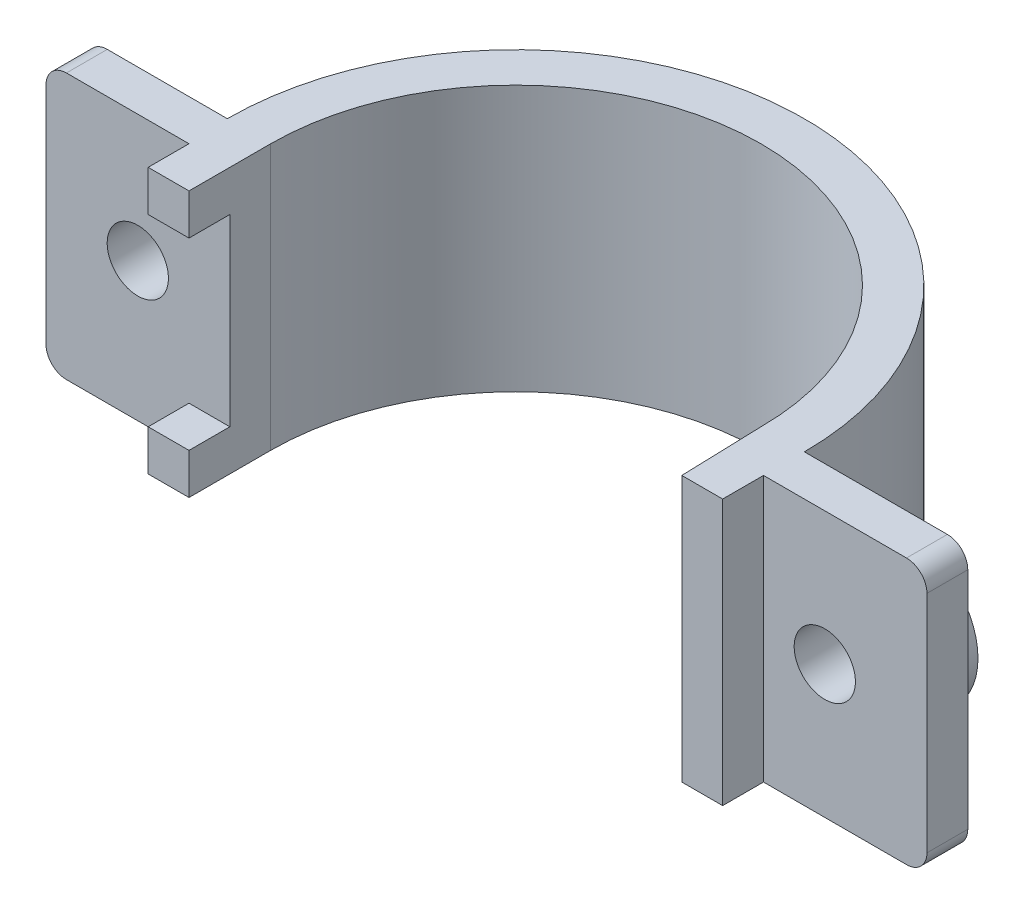
ISO-10303-21;
HEADER;
FILE_DESCRIPTION(('STEP AP214'),'2;1');
FILE_NAME('part.step','',(''),(''),'','','');
FILE_SCHEMA(('AUTOMOTIVE_DESIGN { 1 0 10303 214 1 1 1 1 }'));
ENDSEC;
DATA;
#1=APPLICATION_CONTEXT('core data for automotive mechanical design processes');
#2=APPLICATION_PROTOCOL_DEFINITION('international standard','automotive_design',2000,#1);
#3=PRODUCT_CONTEXT('',#1,'mechanical');
#4=PRODUCT('Part','Part','',(#3));
#5=PRODUCT_RELATED_PRODUCT_CATEGORY('part','',(#4));
#6=PRODUCT_DEFINITION_FORMATION('','',#4);
#7=PRODUCT_DEFINITION_CONTEXT('part definition',#1,'design');
#8=PRODUCT_DEFINITION('design','',#6,#7);
#9=PRODUCT_DEFINITION_SHAPE('','',#8);
#10=(LENGTH_UNIT() NAMED_UNIT(*) SI_UNIT(.MILLI.,.METRE.));
#11=(NAMED_UNIT(*) PLANE_ANGLE_UNIT() SI_UNIT($,.RADIAN.));
#12=(NAMED_UNIT(*) SI_UNIT($,.STERADIAN.) SOLID_ANGLE_UNIT());
#13=UNCERTAINTY_MEASURE_WITH_UNIT(LENGTH_MEASURE(1.E-05),#10,'distance_accuracy_value','');
#14=(GEOMETRIC_REPRESENTATION_CONTEXT(3) GLOBAL_UNCERTAINTY_ASSIGNED_CONTEXT((#13)) GLOBAL_UNIT_ASSIGNED_CONTEXT((#10,
#11,#12)) REPRESENTATION_CONTEXT('',''));
#15=CARTESIAN_POINT('',(0.,0.,0.));
#16=DIRECTION('',(0.,0.,1.));
#17=DIRECTION('',(1.,0.,0.));
#18=AXIS2_PLACEMENT_3D('',#15,#16,#17);
#19=CARTESIAN_POINT('',(165.624085247545,15.,0.));
#20=DIRECTION('',(0.,0.,1.));
#21=DIRECTION('',(1.,0.,0.));
#22=AXIS2_PLACEMENT_3D('',#19,#20,#21);
#23=PLANE('',#22);
#24=DIRECTION('',(1.,0.,0.));
#25=VECTOR('',#24,1.);
#26=CARTESIAN_POINT('',(130.624085247545,60.,0.));
#27=LINE('',#26,#25);
#28=CARTESIAN_POINT('',(130.624085247545,60.,0.));
#29=VERTEX_POINT('',#28);
#30=CARTESIAN_POINT('',(145.624085247545,60.,0.));
#31=VERTEX_POINT('',#30);
#32=EDGE_CURVE('E270',#29,#31,#27,.T.);
#33=ORIENTED_EDGE('',*,*,#32,.F.);
#34=DIRECTION('',(0.,1.,0.));
#35=VECTOR('',#34,1.);
#36=CARTESIAN_POINT('',(130.624085247545,9.99999999999999,0.));
#37=LINE('',#36,#35);
#38=CARTESIAN_POINT('',(130.624085247545,75.,0.));
#39=VERTEX_POINT('',#38);
#40=EDGE_CURVE('E364',#29,#39,#37,.T.);
#41=ORIENTED_EDGE('',*,*,#40,.T.);
#42=DIRECTION('',(-1.,0.,0.));
#43=VECTOR('',#42,1.);
#44=CARTESIAN_POINT('',(130.624085247545,75.,0.));
#45=LINE('',#44,#43);
#46=CARTESIAN_POINT('',(165.624085247545,75.,0.));
#47=VERTEX_POINT('',#46);
#48=EDGE_CURVE('E304',#47,#39,#45,.T.);
#49=ORIENTED_EDGE('',*,*,#48,.F.);
#50=CARTESIAN_POINT('',(165.624085247545,70.,0.));
#51=DIRECTION('',(0.,0.,1.));
#52=DIRECTION('',(1.,0.,0.));
#53=AXIS2_PLACEMENT_3D('',#50,#51,#52);
#54=CIRCLE('',#53,5.00000000000002);
#55=CARTESIAN_POINT('',(170.624085247545,70.,0.));
#56=VERTEX_POINT('',#55);
#57=EDGE_CURVE('E321',#56,#47,#54,.T.);
#58=ORIENTED_EDGE('',*,*,#57,.F.);
#59=DIRECTION('',(0.,1.,0.));
#60=VECTOR('',#59,1.);
#61=CARTESIAN_POINT('',(170.624085247545,70.,0.));
#62=LINE('',#61,#60);
#63=CARTESIAN_POINT('',(170.624085247545,15.,0.));
#64=VERTEX_POINT('',#63);
#65=EDGE_CURVE('E318',#64,#56,#62,.T.);
#66=ORIENTED_EDGE('',*,*,#65,.F.);
#67=CARTESIAN_POINT('',(165.624085247545,15.,0.));
#68=DIRECTION('',(0.,0.,1.));
#69=DIRECTION('',(1.,0.,0.));
#70=AXIS2_PLACEMENT_3D('',#67,#68,#69);
#71=CIRCLE('',#70,5.);
#72=CARTESIAN_POINT('',(165.624085247545,9.99999999999999,0.));
#73=VERTEX_POINT('',#72);
#74=EDGE_CURVE('E319',#73,#64,#71,.T.);
#75=ORIENTED_EDGE('',*,*,#74,.F.);
#76=DIRECTION('',(1.,0.,0.));
#77=VECTOR('',#76,1.);
#78=CARTESIAN_POINT('',(130.624085247545,9.99999999999999,0.));
#79=LINE('',#78,#77);
#80=CARTESIAN_POINT('',(130.624085247545,9.99999999999999,0.));
#81=VERTEX_POINT('',#80);
#82=EDGE_CURVE('E297',#81,#73,#79,.T.);
#83=ORIENTED_EDGE('',*,*,#82,.F.);
#84=CARTESIAN_POINT('',(130.624085247545,25.,0.));
#85=VERTEX_POINT('',#84);
#86=EDGE_CURVE('E374',#81,#85,#37,.T.);
#87=ORIENTED_EDGE('',*,*,#86,.T.);
#88=DIRECTION('',(-1.,0.,0.));
#89=VECTOR('',#88,1.);
#90=CARTESIAN_POINT('',(130.624085247545,25.,0.));
#91=LINE('',#90,#89);
#92=CARTESIAN_POINT('',(145.624085247545,25.,0.));
#93=VERTEX_POINT('',#92);
#94=EDGE_CURVE('E280',#93,#85,#91,.T.);
#95=ORIENTED_EDGE('',*,*,#94,.F.);
#96=CARTESIAN_POINT('',(145.624085247545,42.5,0.));
#97=DIRECTION('',(0.,0.,-1.));
#98=DIRECTION('',(-1.,0.,0.));
#99=AXIS2_PLACEMENT_3D('',#96,#97,#98);
#100=CIRCLE('',#99,17.5);
#101=EDGE_CURVE('E67',#31,#93,#100,.T.);
#102=ORIENTED_EDGE('',*,*,#101,.F.);
#103=EDGE_LOOP('',(#33,#41,#49,#58,#66,#75,#83,#87,#95,#102));
#104=FACE_BOUND('',#103,.T.);
#105=ADVANCED_FACE('F50',(#104),#23,.F.);
#106=CARTESIAN_POINT('',(-40.,15.,10.));
#107=DIRECTION('',(0.,0.,1.));
#108=DIRECTION('',(1.,0.,0.));
#109=AXIS2_PLACEMENT_3D('',#106,#107,#108);
#110=PLANE('',#109);
#111=CARTESIAN_POINT('',(-22.530823522442,43.9464892567154,10.));
#112=DIRECTION('',(0.,0.,-1.));
#113=DIRECTION('',(-1.,0.,0.));
#114=AXIS2_PLACEMENT_3D('',#111,#112,#113);
#115=CIRCLE('',#114,7.5);
#116=CARTESIAN_POINT('',(-30.030823522442,43.9464892567154,10.));
#117=VERTEX_POINT('',#116);
#118=EDGE_CURVE('E631',#117,#117,#115,.T.);
#119=ORIENTED_EDGE('',*,*,#118,.T.);
#120=EDGE_LOOP('',(#119));
#121=FACE_BOUND('',#120,.T.);
#122=DIRECTION('',(0.,-1.,0.));
#123=VECTOR('',#122,1.);
#124=CARTESIAN_POINT('',(-10.,20.,10.));
#125=LINE('',#124,#123);
#126=CARTESIAN_POINT('',(-10.,20.,10.));
#127=VERTEX_POINT('',#126);
#128=CARTESIAN_POINT('',(-10.,10.,10.));
#129=VERTEX_POINT('',#128);
#130=EDGE_CURVE('E382',#127,#129,#125,.T.);
#131=ORIENTED_EDGE('',*,*,#130,.F.);
#132=DIRECTION('',(-1.,0.,0.));
#133=VECTOR('',#132,1.);
#134=CARTESIAN_POINT('',(0.,20.,10.));
#135=LINE('',#134,#133);
#136=CARTESIAN_POINT('',(0.,20.,10.));
#137=VERTEX_POINT('',#136);
#138=EDGE_CURVE('E369',#137,#127,#135,.T.);
#139=ORIENTED_EDGE('',*,*,#138,.F.);
#140=DIRECTION('',(0.,1.,0.));
#141=VECTOR('',#140,1.);
#142=CARTESIAN_POINT('',(0.,75.,10.));
#143=LINE('',#142,#141);
#144=CARTESIAN_POINT('',(0.,65.,10.));
#145=VERTEX_POINT('',#144);
#146=EDGE_CURVE('E422',#137,#145,#143,.T.);
#147=ORIENTED_EDGE('',*,*,#146,.T.);
#148=DIRECTION('',(1.,0.,0.));
#149=VECTOR('',#148,1.);
#150=CARTESIAN_POINT('',(-10.,65.,10.));
#151=LINE('',#150,#149);
#152=CARTESIAN_POINT('',(-10.,65.,10.));
#153=VERTEX_POINT('',#152);
#154=EDGE_CURVE('E405',#153,#145,#151,.T.);
#155=ORIENTED_EDGE('',*,*,#154,.F.);
#156=DIRECTION('',(0.,-1.,0.));
#157=VECTOR('',#156,1.);
#158=CARTESIAN_POINT('',(-10.,75.,10.));
#159=LINE('',#158,#157);
#160=CARTESIAN_POINT('',(-10.,75.,10.));
#161=VERTEX_POINT('',#160);
#162=EDGE_CURVE('E396',#161,#153,#159,.T.);
#163=ORIENTED_EDGE('',*,*,#162,.F.);
#164=DIRECTION('',(-1.,0.,0.));
#165=VECTOR('',#164,1.);
#166=CARTESIAN_POINT('',(0.,75.,10.));
#167=LINE('',#166,#165);
#168=CARTESIAN_POINT('',(-40.,75.,10.));
#169=VERTEX_POINT('',#168);
#170=EDGE_CURVE('E425',#161,#169,#167,.T.);
#171=ORIENTED_EDGE('',*,*,#170,.T.);
#172=CARTESIAN_POINT('',(-40.,70.,10.));
#173=DIRECTION('',(0.,0.,1.));
#174=DIRECTION('',(1.,0.,0.));
#175=AXIS2_PLACEMENT_3D('',#172,#173,#174);
#176=CIRCLE('',#175,5.);
#177=CARTESIAN_POINT('',(-45.,70.,10.));
#178=VERTEX_POINT('',#177);
#179=EDGE_CURVE('E430',#169,#178,#176,.T.);
#180=ORIENTED_EDGE('',*,*,#179,.T.);
#181=DIRECTION('',(0.,-1.,0.));
#182=VECTOR('',#181,1.);
#183=CARTESIAN_POINT('',(-45.,70.,10.));
#184=LINE('',#183,#182);
#185=CARTESIAN_POINT('',(-45.,15.,10.));
#186=VERTEX_POINT('',#185);
#187=EDGE_CURVE('E429',#178,#186,#184,.T.);
#188=ORIENTED_EDGE('',*,*,#187,.T.);
#189=CARTESIAN_POINT('',(-40.,15.,10.));
#190=DIRECTION('',(0.,0.,1.));
#191=DIRECTION('',(1.,0.,0.));
#192=AXIS2_PLACEMENT_3D('',#189,#190,#191);
#193=CIRCLE('',#192,5.);
#194=CARTESIAN_POINT('',(-40.,10.,10.));
#195=VERTEX_POINT('',#194);
#196=EDGE_CURVE('E431',#186,#195,#193,.T.);
#197=ORIENTED_EDGE('',*,*,#196,.T.);
#198=DIRECTION('',(1.,0.,0.));
#199=VECTOR('',#198,1.);
#200=CARTESIAN_POINT('',(0.,10.,10.));
#201=LINE('',#200,#199);
#202=EDGE_CURVE('E433',#195,#129,#201,.T.);
#203=ORIENTED_EDGE('',*,*,#202,.T.);
#204=EDGE_LOOP('',(#131,#139,#147,#155,#163,#171,#180,#188,#197,#203));
#205=FACE_BOUND('',#204,.T.);
#206=ADVANCED_FACE('F482',(#121,#205),#110,.T.);
#207=CARTESIAN_POINT('',(0.,75.,10.));
#208=DIRECTION('',(-1.,0.,0.));
#209=DIRECTION('',(0.,0.,1.));
#210=AXIS2_PLACEMENT_3D('',#207,#208,#209);
#211=PLANE('',#210);
#212=DIRECTION('',(0.,1.,0.));
#213=VECTOR('',#212,1.);
#214=CARTESIAN_POINT('',(0.,75.,0.));
#215=LINE('',#214,#213);
#216=CARTESIAN_POINT('',(0.,9.99999999999999,0.));
#217=VERTEX_POINT('',#216);
#218=CARTESIAN_POINT('',(0.,75.,0.));
#219=VERTEX_POINT('',#218);
#220=EDGE_CURVE('E423',#217,#219,#215,.T.);
#221=ORIENTED_EDGE('',*,*,#220,.T.);
#222=DIRECTION('',(0.,0.,-1.));
#223=VECTOR('',#222,1.);
#224=CARTESIAN_POINT('',(0.,75.,10.));
#225=LINE('',#224,#223);
#226=CARTESIAN_POINT('',(0.,75.,20.));
#227=VERTEX_POINT('',#226);
#228=EDGE_CURVE('E11',#227,#219,#225,.T.);
#229=ORIENTED_EDGE('',*,*,#228,.F.);
#230=DIRECTION('',(0.,1.,0.));
#231=VECTOR('',#230,1.);
#232=CARTESIAN_POINT('',(0.,65.,20.));
#233=LINE('',#232,#231);
#234=CARTESIAN_POINT('',(0.,65.,20.));
#235=VERTEX_POINT('',#234);
#236=EDGE_CURVE('E400',#235,#227,#233,.T.);
#237=ORIENTED_EDGE('',*,*,#236,.F.);
#238=DIRECTION('',(0.,0.,-1.));
#239=VECTOR('',#238,1.);
#240=CARTESIAN_POINT('',(0.,65.,20.));
#241=LINE('',#240,#239);
#242=EDGE_CURVE('E410',#235,#145,#241,.T.);
#243=ORIENTED_EDGE('',*,*,#242,.T.);
#244=ORIENTED_EDGE('',*,*,#146,.F.);
#245=DIRECTION('',(0.,0.,-1.));
#246=VECTOR('',#245,1.);
#247=CARTESIAN_POINT('',(0.,20.,20.));
#248=LINE('',#247,#246);
#249=CARTESIAN_POINT('',(0.,20.,20.));
#250=VERTEX_POINT('',#249);
#251=EDGE_CURVE('E392',#250,#137,#248,.T.);
#252=ORIENTED_EDGE('',*,*,#251,.F.);
#253=DIRECTION('',(0.,1.,0.));
#254=VECTOR('',#253,1.);
#255=CARTESIAN_POINT('',(0.,10.,20.));
#256=LINE('',#255,#254);
#257=CARTESIAN_POINT('',(0.,10.,20.));
#258=VERTEX_POINT('',#257);
#259=EDGE_CURVE('E379',#258,#250,#256,.T.);
#260=ORIENTED_EDGE('',*,*,#259,.F.);
#261=DIRECTION('',(0.,0.,-1.));
#262=VECTOR('',#261,1.);
#263=CARTESIAN_POINT('',(0.,10.,10.));
#264=LINE('',#263,#262);
#265=EDGE_CURVE('E436',#258,#217,#264,.T.);
#266=ORIENTED_EDGE('',*,*,#265,.T.);
#267=EDGE_LOOP('',(#221,#229,#237,#243,#244,#252,#260,#266));
#268=FACE_BOUND('',#267,.T.);
#269=ADVANCED_FACE('F47',(#268),#211,.F.);
#270=CARTESIAN_POINT('',(0.,75.,10.));
#271=DIRECTION('',(0.,-1.,0.));
#272=DIRECTION('',(0.,0.,-1.));
#273=AXIS2_PLACEMENT_3D('',#270,#271,#272);
#274=PLANE('',#273);
#275=ORIENTED_EDGE('',*,*,#228,.T.);
#276=CARTESIAN_POINT('',(60.,75.,0.));
#277=DIRECTION('',(0.,1.,0.));
#278=DIRECTION('',(0.,0.,1.));
#279=AXIS2_PLACEMENT_3D('',#276,#277,#278);
#280=CIRCLE('',#279,60.);
#281=CARTESIAN_POINT('',(120.,75.,0.));
#282=VERTEX_POINT('',#281);
#283=EDGE_CURVE('E365',#282,#219,#280,.T.);
#284=ORIENTED_EDGE('',*,*,#283,.F.);
#285=DIRECTION('',(0.0311890815739658,0.,0.999513502255259));
#286=VECTOR('',#285,1.);
#287=CARTESIAN_POINT('',(120.624085247545,75.,20.));
#288=LINE('',#287,#286);
#289=CARTESIAN_POINT('',(120.624085247545,75.,20.));
#290=VERTEX_POINT('',#289);
#291=EDGE_CURVE('E340',#282,#290,#288,.T.);
#292=ORIENTED_EDGE('',*,*,#291,.T.);
#293=DIRECTION('',(1.,0.,0.));
#294=VECTOR('',#293,1.);
#295=CARTESIAN_POINT('',(130.624085247545,75.,20.));
#296=LINE('',#295,#294);
#297=CARTESIAN_POINT('',(130.624085247545,75.,20.));
#298=VERTEX_POINT('',#297);
#299=EDGE_CURVE('E347',#290,#298,#296,.T.);
#300=ORIENTED_EDGE('',*,*,#299,.T.);
#301=DIRECTION('',(0.,0.,-1.));
#302=VECTOR('',#301,1.);
#303=CARTESIAN_POINT('',(130.624085247545,75.,0.));
#304=LINE('',#303,#302);
#305=CARTESIAN_POINT('',(130.624085247545,75.,10.));
#306=VERTEX_POINT('',#305);
#307=EDGE_CURVE('E341',#298,#306,#304,.T.);
#308=ORIENTED_EDGE('',*,*,#307,.T.);
#309=DIRECTION('',(-1.,0.,0.));
#310=VECTOR('',#309,1.);
#311=CARTESIAN_POINT('',(130.624085247545,75.,10.));
#312=LINE('',#311,#310);
#313=CARTESIAN_POINT('',(165.624085247545,75.,10.));
#314=VERTEX_POINT('',#313);
#315=EDGE_CURVE('E312',#314,#306,#312,.T.);
#316=ORIENTED_EDGE('',*,*,#315,.F.);
#317=DIRECTION('',(0.,0.,-1.));
#318=VECTOR('',#317,1.);
#319=CARTESIAN_POINT('',(165.624085247545,75.,10.));
#320=LINE('',#319,#318);
#321=EDGE_CURVE('E317',#314,#47,#320,.T.);
#322=ORIENTED_EDGE('',*,*,#321,.T.);
#323=ORIENTED_EDGE('',*,*,#48,.T.);
#324=CARTESIAN_POINT('',(60.,75.,0.));
#325=DIRECTION('',(0.,1.,0.));
#326=DIRECTION('',(0.,0.,1.));
#327=AXIS2_PLACEMENT_3D('',#324,#325,#326);
#328=CIRCLE('',#327,70.6240852475448);
#329=CARTESIAN_POINT('',(-10.6240852475448,75.,0.));
#330=VERTEX_POINT('',#329);
#331=EDGE_CURVE('E357',#39,#330,#328,.T.);
#332=ORIENTED_EDGE('',*,*,#331,.T.);
#333=DIRECTION('',(-1.,0.,0.));
#334=VECTOR('',#333,1.);
#335=CARTESIAN_POINT('',(0.,75.,0.));
#336=LINE('',#335,#334);
#337=CARTESIAN_POINT('',(-40.,75.,0.));
#338=VERTEX_POINT('',#337);
#339=EDGE_CURVE('E437',#330,#338,#336,.T.);
#340=ORIENTED_EDGE('',*,*,#339,.T.);
#341=DIRECTION('',(0.,0.,-1.));
#342=VECTOR('',#341,1.);
#343=CARTESIAN_POINT('',(-40.,75.,10.));
#344=LINE('',#343,#342);
#345=EDGE_CURVE('E54',#169,#338,#344,.T.);
#346=ORIENTED_EDGE('',*,*,#345,.F.);
#347=ORIENTED_EDGE('',*,*,#170,.F.);
#348=DIRECTION('',(0.,0.,-1.));
#349=VECTOR('',#348,1.);
#350=CARTESIAN_POINT('',(-10.,75.,20.));
#351=LINE('',#350,#349);
#352=CARTESIAN_POINT('',(-10.,75.,20.));
#353=VERTEX_POINT('',#352);
#354=EDGE_CURVE('E420',#353,#161,#351,.T.);
#355=ORIENTED_EDGE('',*,*,#354,.F.);
#356=DIRECTION('',(-1.,0.,0.));
#357=VECTOR('',#356,1.);
#358=CARTESIAN_POINT('',(0.,75.,20.));
#359=LINE('',#358,#357);
#360=EDGE_CURVE('E402',#227,#353,#359,.T.);
#361=ORIENTED_EDGE('',*,*,#360,.F.);
#362=EDGE_LOOP('',(#275,#284,#292,#300,#308,#316,#322,#323,#332,#340,#346,#347,#355,#361));
#363=FACE_BOUND('',#362,.T.);
#364=ADVANCED_FACE('F487',(#363),#274,.F.);
#365=CARTESIAN_POINT('',(-40.,70.,10.));
#366=DIRECTION('',(0.,0.,-1.));
#367=DIRECTION('',(-1.,0.,0.));
#368=AXIS2_PLACEMENT_3D('',#365,#366,#367);
#369=CYLINDRICAL_SURFACE('',#368,5.);
#370=CARTESIAN_POINT('',(-40.,70.,0.));
#371=DIRECTION('',(0.,0.,1.));
#372=DIRECTION('',(1.,0.,0.));
#373=AXIS2_PLACEMENT_3D('',#370,#371,#372);
#374=CIRCLE('',#373,5.);
#375=CARTESIAN_POINT('',(-45.,70.,0.));
#376=VERTEX_POINT('',#375);
#377=EDGE_CURVE('E441',#338,#376,#374,.T.);
#378=ORIENTED_EDGE('',*,*,#377,.T.);
#379=DIRECTION('',(0.,0.,-1.));
#380=VECTOR('',#379,1.);
#381=CARTESIAN_POINT('',(-45.,70.,10.));
#382=LINE('',#381,#380);
#383=EDGE_CURVE('E460',#178,#376,#382,.T.);
#384=ORIENTED_EDGE('',*,*,#383,.F.);
#385=ORIENTED_EDGE('',*,*,#179,.F.);
#386=ORIENTED_EDGE('',*,*,#345,.T.);
#387=EDGE_LOOP('',(#378,#384,#385,#386));
#388=FACE_BOUND('',#387,.T.);
#389=ADVANCED_FACE('F463',(#388),#369,.T.);
#390=CARTESIAN_POINT('',(-45.,70.,10.));
#391=DIRECTION('',(1.,0.,0.));
#392=DIRECTION('',(0.,0.,-1.));
#393=AXIS2_PLACEMENT_3D('',#390,#391,#392);
#394=PLANE('',#393);
#395=DIRECTION('',(0.,-1.,0.));
#396=VECTOR('',#395,1.);
#397=CARTESIAN_POINT('',(-45.,70.,0.));
#398=LINE('',#397,#396);
#399=CARTESIAN_POINT('',(-45.,15.,0.));
#400=VERTEX_POINT('',#399);
#401=EDGE_CURVE('E442',#376,#400,#398,.T.);
#402=ORIENTED_EDGE('',*,*,#401,.T.);
#403=DIRECTION('',(0.,0.,-1.));
#404=VECTOR('',#403,1.);
#405=CARTESIAN_POINT('',(-45.,15.,10.));
#406=LINE('',#405,#404);
#407=EDGE_CURVE('E453',#186,#400,#406,.T.);
#408=ORIENTED_EDGE('',*,*,#407,.F.);
#409=ORIENTED_EDGE('',*,*,#187,.F.);
#410=ORIENTED_EDGE('',*,*,#383,.T.);
#411=EDGE_LOOP('',(#402,#408,#409,#410));
#412=FACE_BOUND('',#411,.T.);
#413=ADVANCED_FACE('F478',(#412),#394,.F.);
#414=CARTESIAN_POINT('',(-40.,15.,10.));
#415=DIRECTION('',(0.,0.,-1.));
#416=DIRECTION('',(-1.,0.,0.));
#417=AXIS2_PLACEMENT_3D('',#414,#415,#416);
#418=CYLINDRICAL_SURFACE('',#417,5.);
#419=CARTESIAN_POINT('',(-40.,15.,0.));
#420=DIRECTION('',(0.,0.,1.));
#421=DIRECTION('',(1.,0.,0.));
#422=AXIS2_PLACEMENT_3D('',#419,#420,#421);
#423=CIRCLE('',#422,5.);
#424=CARTESIAN_POINT('',(-40.,10.,0.));
#425=VERTEX_POINT('',#424);
#426=EDGE_CURVE('E444',#400,#425,#423,.T.);
#427=ORIENTED_EDGE('',*,*,#426,.T.);
#428=DIRECTION('',(0.,0.,-1.));
#429=VECTOR('',#428,1.);
#430=CARTESIAN_POINT('',(-40.,10.,10.));
#431=LINE('',#430,#429);
#432=EDGE_CURVE('E454',#195,#425,#431,.T.);
#433=ORIENTED_EDGE('',*,*,#432,.F.);
#434=ORIENTED_EDGE('',*,*,#196,.F.);
#435=ORIENTED_EDGE('',*,*,#407,.T.);
#436=EDGE_LOOP('',(#427,#433,#434,#435));
#437=FACE_BOUND('',#436,.T.);
#438=ADVANCED_FACE('F477',(#437),#418,.T.);
#439=CARTESIAN_POINT('',(0.,10.,10.));
#440=DIRECTION('',(0.,1.,0.));
#441=DIRECTION('',(0.,0.,1.));
#442=AXIS2_PLACEMENT_3D('',#439,#440,#441);
#443=PLANE('',#442);
#444=DIRECTION('',(1.,0.,0.));
#445=VECTOR('',#444,1.);
#446=CARTESIAN_POINT('',(0.,10.,0.));
#447=LINE('',#446,#445);
#448=CARTESIAN_POINT('',(-10.6240852475448,9.99999999999999,0.));
#449=VERTEX_POINT('',#448);
#450=EDGE_CURVE('E424',#425,#449,#447,.T.);
#451=ORIENTED_EDGE('',*,*,#450,.T.);
#452=CARTESIAN_POINT('',(60.,9.99999999999999,0.));
#453=DIRECTION('',(0.,1.,0.));
#454=DIRECTION('',(0.,0.,1.));
#455=AXIS2_PLACEMENT_3D('',#452,#453,#454);
#456=CIRCLE('',#455,70.6240852475448);
#457=EDGE_CURVE('E360',#81,#449,#456,.T.);
#458=ORIENTED_EDGE('',*,*,#457,.F.);
#459=ORIENTED_EDGE('',*,*,#82,.T.);
#460=DIRECTION('',(0.,0.,-1.));
#461=VECTOR('',#460,1.);
#462=CARTESIAN_POINT('',(165.624085247545,9.99999999999999,10.));
#463=LINE('',#462,#461);
#464=CARTESIAN_POINT('',(165.624085247545,9.99999999999999,10.));
#465=VERTEX_POINT('',#464);
#466=EDGE_CURVE('E333',#465,#73,#463,.T.);
#467=ORIENTED_EDGE('',*,*,#466,.F.);
#468=DIRECTION('',(1.,0.,0.));
#469=VECTOR('',#468,1.);
#470=CARTESIAN_POINT('',(130.624085247545,9.99999999999999,10.));
#471=LINE('',#470,#469);
#472=CARTESIAN_POINT('',(130.624085247545,9.99999999999999,10.));
#473=VERTEX_POINT('',#472);
#474=EDGE_CURVE('E302',#473,#465,#471,.T.);
#475=ORIENTED_EDGE('',*,*,#474,.F.);
#476=DIRECTION('',(0.,0.,-1.));
#477=VECTOR('',#476,1.);
#478=CARTESIAN_POINT('',(130.624085247545,9.99999999999999,0.));
#479=LINE('',#478,#477);
#480=CARTESIAN_POINT('',(130.624085247545,9.99999999999999,20.));
#481=VERTEX_POINT('',#480);
#482=EDGE_CURVE('E342',#481,#473,#479,.T.);
#483=ORIENTED_EDGE('',*,*,#482,.F.);
#484=DIRECTION('',(1.,0.,0.));
#485=VECTOR('',#484,1.);
#486=CARTESIAN_POINT('',(130.624085247545,9.99999999999999,20.));
#487=LINE('',#486,#485);
#488=CARTESIAN_POINT('',(120.624085247545,9.99999999999999,20.));
#489=VERTEX_POINT('',#488);
#490=EDGE_CURVE('E344',#489,#481,#487,.T.);
#491=ORIENTED_EDGE('',*,*,#490,.F.);
#492=DIRECTION('',(0.0311890815739658,0.,0.999513502255259));
#493=VECTOR('',#492,1.);
#494=CARTESIAN_POINT('',(120.624085247545,9.99999999999999,20.));
#495=LINE('',#494,#493);
#496=CARTESIAN_POINT('',(120.,9.99999999999999,0.));
#497=VERTEX_POINT('',#496);
#498=EDGE_CURVE('E336',#497,#489,#495,.T.);
#499=ORIENTED_EDGE('',*,*,#498,.F.);
#500=CARTESIAN_POINT('',(60.,9.99999999999999,0.));
#501=DIRECTION('',(0.,1.,0.));
#502=DIRECTION('',(0.,0.,1.));
#503=AXIS2_PLACEMENT_3D('',#500,#501,#502);
#504=CIRCLE('',#503,60.);
#505=EDGE_CURVE('E363',#497,#217,#504,.T.);
#506=ORIENTED_EDGE('',*,*,#505,.T.);
#507=ORIENTED_EDGE('',*,*,#265,.F.);
#508=DIRECTION('',(1.,0.,0.));
#509=VECTOR('',#508,1.);
#510=CARTESIAN_POINT('',(-10.,10.,20.));
#511=LINE('',#510,#509);
#512=CARTESIAN_POINT('',(-10.,10.,20.));
#513=VERTEX_POINT('',#512);
#514=EDGE_CURVE('E380',#513,#258,#511,.T.);
#515=ORIENTED_EDGE('',*,*,#514,.F.);
#516=DIRECTION('',(0.,0.,-1.));
#517=VECTOR('',#516,1.);
#518=CARTESIAN_POINT('',(-10.,10.,20.));
#519=LINE('',#518,#517);
#520=EDGE_CURVE('E386',#513,#129,#519,.T.);
#521=ORIENTED_EDGE('',*,*,#520,.T.);
#522=ORIENTED_EDGE('',*,*,#202,.F.);
#523=ORIENTED_EDGE('',*,*,#432,.T.);
#524=EDGE_LOOP('',(#451,#458,#459,#467,#475,#483,#491,#499,#506,#507,#515,#521,#522,#523));
#525=FACE_BOUND('',#524,.T.);
#526=ADVANCED_FACE('F512',(#525),#443,.F.);
#527=CARTESIAN_POINT('',(-40.,15.,0.));
#528=DIRECTION('',(0.,0.,1.));
#529=DIRECTION('',(1.,0.,0.));
#530=AXIS2_PLACEMENT_3D('',#527,#528,#529);
#531=PLANE('',#530);
#532=DIRECTION('',(1.,0.,0.));
#533=VECTOR('',#532,1.);
#534=CARTESIAN_POINT('',(-10.6240852475448,60.,0.));
#535=LINE('',#534,#533);
#536=CARTESIAN_POINT('',(-20.6240852475448,60.,0.));
#537=VERTEX_POINT('',#536);
#538=CARTESIAN_POINT('',(-10.6240852475448,60.,0.));
#539=VERTEX_POINT('',#538);
#540=EDGE_CURVE('E61',#537,#539,#535,.T.);
#541=ORIENTED_EDGE('',*,*,#540,.F.);
#542=CARTESIAN_POINT('',(-20.6240852475448,42.5,0.));
#543=DIRECTION('',(0.,0.,-1.));
#544=DIRECTION('',(-1.,0.,0.));
#545=AXIS2_PLACEMENT_3D('',#542,#543,#544);
#546=CIRCLE('',#545,17.5);
#547=CARTESIAN_POINT('',(-20.6240852475448,25.,0.));
#548=VERTEX_POINT('',#547);
#549=EDGE_CURVE('E265',#548,#537,#546,.T.);
#550=ORIENTED_EDGE('',*,*,#549,.F.);
#551=DIRECTION('',(-1.,0.,0.));
#552=VECTOR('',#551,1.);
#553=CARTESIAN_POINT('',(-20.6240852475448,25.,0.));
#554=LINE('',#553,#552);
#555=CARTESIAN_POINT('',(-10.6240852475448,25.,0.));
#556=VERTEX_POINT('',#555);
#557=EDGE_CURVE('E543',#556,#548,#554,.T.);
#558=ORIENTED_EDGE('',*,*,#557,.F.);
#559=DIRECTION('',(0.,1.,0.));
#560=VECTOR('',#559,1.);
#561=CARTESIAN_POINT('',(-10.6240852475448,9.99999999999999,0.));
#562=LINE('',#561,#560);
#563=EDGE_CURVE('E371',#449,#556,#562,.T.);
#564=ORIENTED_EDGE('',*,*,#563,.F.);
#565=ORIENTED_EDGE('',*,*,#450,.F.);
#566=ORIENTED_EDGE('',*,*,#426,.F.);
#567=ORIENTED_EDGE('',*,*,#401,.F.);
#568=ORIENTED_EDGE('',*,*,#377,.F.);
#569=ORIENTED_EDGE('',*,*,#339,.F.);
#570=EDGE_CURVE('E372',#539,#330,#562,.T.);
#571=ORIENTED_EDGE('',*,*,#570,.F.);
#572=EDGE_LOOP('',(#541,#550,#558,#564,#565,#566,#567,#568,#569,#571));
#573=FACE_BOUND('',#572,.T.);
#574=ADVANCED_FACE('F474',(#573),#531,.F.);
#575=CARTESIAN_POINT('',(-10.,75.,20.));
#576=DIRECTION('',(1.,0.,0.));
#577=DIRECTION('',(0.,0.,-1.));
#578=AXIS2_PLACEMENT_3D('',#575,#576,#577);
#579=PLANE('',#578);
#580=ORIENTED_EDGE('',*,*,#162,.T.);
#581=DIRECTION('',(0.,0.,-1.));
#582=VECTOR('',#581,1.);
#583=CARTESIAN_POINT('',(-10.,65.,20.));
#584=LINE('',#583,#582);
#585=CARTESIAN_POINT('',(-10.,65.,20.));
#586=VERTEX_POINT('',#585);
#587=EDGE_CURVE('E412',#586,#153,#584,.T.);
#588=ORIENTED_EDGE('',*,*,#587,.F.);
#589=DIRECTION('',(0.,-1.,0.));
#590=VECTOR('',#589,1.);
#591=CARTESIAN_POINT('',(-10.,75.,20.));
#592=LINE('',#591,#590);
#593=EDGE_CURVE('E404',#353,#586,#592,.T.);
#594=ORIENTED_EDGE('',*,*,#593,.F.);
#595=ORIENTED_EDGE('',*,*,#354,.T.);
#596=EDGE_LOOP('',(#580,#588,#594,#595));
#597=FACE_BOUND('',#596,.T.);
#598=ADVANCED_FACE('F493',(#597),#579,.F.);
#599=CARTESIAN_POINT('',(-10.,65.,20.));
#600=DIRECTION('',(0.,1.,0.));
#601=DIRECTION('',(0.,0.,1.));
#602=AXIS2_PLACEMENT_3D('',#599,#600,#601);
#603=PLANE('',#602);
#604=ORIENTED_EDGE('',*,*,#154,.T.);
#605=ORIENTED_EDGE('',*,*,#242,.F.);
#606=DIRECTION('',(1.,0.,0.));
#607=VECTOR('',#606,1.);
#608=CARTESIAN_POINT('',(-10.,65.,20.));
#609=LINE('',#608,#607);
#610=EDGE_CURVE('E409',#586,#235,#609,.T.);
#611=ORIENTED_EDGE('',*,*,#610,.F.);
#612=ORIENTED_EDGE('',*,*,#587,.T.);
#613=EDGE_LOOP('',(#604,#605,#611,#612));
#614=FACE_BOUND('',#613,.T.);
#615=ADVANCED_FACE('F822',(#614),#603,.F.);
#616=CARTESIAN_POINT('',(0.,0.,20.));
#617=DIRECTION('',(0.,0.,1.));
#618=DIRECTION('',(1.,0.,0.));
#619=AXIS2_PLACEMENT_3D('',#616,#617,#618);
#620=PLANE('',#619);
#621=ORIENTED_EDGE('',*,*,#236,.T.);
#622=ORIENTED_EDGE('',*,*,#360,.T.);
#623=ORIENTED_EDGE('',*,*,#593,.T.);
#624=ORIENTED_EDGE('',*,*,#610,.T.);
#625=EDGE_LOOP('',(#621,#622,#623,#624));
#626=FACE_BOUND('',#625,.T.);
#627=ADVANCED_FACE('F492',(#626),#620,.T.);
#628=CARTESIAN_POINT('',(0.,20.,20.));
#629=DIRECTION('',(0.,-1.,0.));
#630=DIRECTION('',(0.,0.,-1.));
#631=AXIS2_PLACEMENT_3D('',#628,#629,#630);
#632=PLANE('',#631);
#633=ORIENTED_EDGE('',*,*,#138,.T.);
#634=DIRECTION('',(0.,0.,-1.));
#635=VECTOR('',#634,1.);
#636=CARTESIAN_POINT('',(-10.,20.,20.));
#637=LINE('',#636,#635);
#638=CARTESIAN_POINT('',(-10.,20.,20.));
#639=VERTEX_POINT('',#638);
#640=EDGE_CURVE('E391',#639,#127,#637,.T.);
#641=ORIENTED_EDGE('',*,*,#640,.F.);
#642=DIRECTION('',(-1.,0.,0.));
#643=VECTOR('',#642,1.);
#644=CARTESIAN_POINT('',(0.,20.,20.));
#645=LINE('',#644,#643);
#646=EDGE_CURVE('E384',#250,#639,#645,.T.);
#647=ORIENTED_EDGE('',*,*,#646,.F.);
#648=ORIENTED_EDGE('',*,*,#251,.T.);
#649=EDGE_LOOP('',(#633,#641,#647,#648));
#650=FACE_BOUND('',#649,.T.);
#651=ADVANCED_FACE('F806',(#650),#632,.F.);
#652=CARTESIAN_POINT('',(-10.,20.,20.));
#653=DIRECTION('',(1.,0.,0.));
#654=DIRECTION('',(0.,0.,-1.));
#655=AXIS2_PLACEMENT_3D('',#652,#653,#654);
#656=PLANE('',#655);
#657=ORIENTED_EDGE('',*,*,#130,.T.);
#658=ORIENTED_EDGE('',*,*,#520,.F.);
#659=DIRECTION('',(0.,-1.,0.));
#660=VECTOR('',#659,1.);
#661=CARTESIAN_POINT('',(-10.,20.,20.));
#662=LINE('',#661,#660);
#663=EDGE_CURVE('E383',#639,#513,#662,.T.);
#664=ORIENTED_EDGE('',*,*,#663,.F.);
#665=ORIENTED_EDGE('',*,*,#640,.T.);
#666=EDGE_LOOP('',(#657,#658,#664,#665));
#667=FACE_BOUND('',#666,.T.);
#668=ADVANCED_FACE('F796',(#667),#656,.F.);
#669=CARTESIAN_POINT('',(0.,0.,20.));
#670=DIRECTION('',(0.,0.,1.));
#671=DIRECTION('',(1.,0.,0.));
#672=AXIS2_PLACEMENT_3D('',#669,#670,#671);
#673=PLANE('',#672);
#674=ORIENTED_EDGE('',*,*,#514,.T.);
#675=ORIENTED_EDGE('',*,*,#259,.T.);
#676=ORIENTED_EDGE('',*,*,#646,.T.);
#677=ORIENTED_EDGE('',*,*,#663,.T.);
#678=EDGE_LOOP('',(#674,#675,#676,#677));
#679=FACE_BOUND('',#678,.T.);
#680=ADVANCED_FACE('F790',(#679),#673,.T.);
#681=CARTESIAN_POINT('',(60.,9.99999999999999,0.));
#682=DIRECTION('',(0.,1.,0.));
#683=DIRECTION('',(0.,0.,1.));
#684=AXIS2_PLACEMENT_3D('',#681,#682,#683);
#685=CYLINDRICAL_SURFACE('',#684,60.);
#686=ORIENTED_EDGE('',*,*,#283,.T.);
#687=ORIENTED_EDGE('',*,*,#220,.F.);
#688=ORIENTED_EDGE('',*,*,#505,.F.);
#689=DIRECTION('',(0.,1.,0.));
#690=VECTOR('',#689,1.);
#691=CARTESIAN_POINT('',(120.,9.99999999999999,0.));
#692=LINE('',#691,#690);
#693=EDGE_CURVE('E368',#497,#282,#692,.T.);
#694=ORIENTED_EDGE('',*,*,#693,.T.);
#695=EDGE_LOOP('',(#686,#687,#688,#694));
#696=FACE_BOUND('',#695,.T.);
#697=ADVANCED_FACE('F502',(#696),#685,.F.);
#698=CARTESIAN_POINT('',(60.,9.99999999999999,0.));
#699=DIRECTION('',(0.,1.,0.));
#700=DIRECTION('',(0.,0.,1.));
#701=AXIS2_PLACEMENT_3D('',#698,#699,#700);
#702=CYLINDRICAL_SURFACE('',#701,70.6240852475448);
#703=ORIENTED_EDGE('',*,*,#331,.F.);
#704=ORIENTED_EDGE('',*,*,#40,.F.);
#705=DIRECTION('',(0.,1.,0.));
#706=VECTOR('',#705,1.);
#707=CARTESIAN_POINT('',(130.624085247545,60.,0.));
#708=LINE('',#707,#706);
#709=EDGE_CURVE('E262',#85,#29,#708,.T.);
#710=ORIENTED_EDGE('',*,*,#709,.F.);
#711=ORIENTED_EDGE('',*,*,#86,.F.);
#712=ORIENTED_EDGE('',*,*,#457,.T.);
#713=ORIENTED_EDGE('',*,*,#563,.T.);
#714=DIRECTION('',(0.,-1.,0.));
#715=VECTOR('',#714,1.);
#716=CARTESIAN_POINT('',(-10.6240852475448,60.,0.));
#717=LINE('',#716,#715);
#718=EDGE_CURVE('E539',#539,#556,#717,.T.);
#719=ORIENTED_EDGE('',*,*,#718,.F.);
#720=ORIENTED_EDGE('',*,*,#570,.T.);
#721=EDGE_LOOP('',(#703,#704,#710,#711,#712,#713,#719,#720));
#722=FACE_BOUND('',#721,.T.);
#723=ADVANCED_FACE('F534',(#722),#702,.T.);
#724=CARTESIAN_POINT('',(130.624085247545,9.99999999999999,0.));
#725=DIRECTION('',(1.,0.,0.));
#726=DIRECTION('',(0.,0.,-1.));
#727=AXIS2_PLACEMENT_3D('',#724,#725,#726);
#728=PLANE('',#727);
#729=DIRECTION('',(0.,-1.,0.));
#730=VECTOR('',#729,1.);
#731=CARTESIAN_POINT('',(130.624085247545,75.,10.));
#732=LINE('',#731,#730);
#733=EDGE_CURVE('E301',#306,#473,#732,.T.);
#734=ORIENTED_EDGE('',*,*,#733,.F.);
#735=ORIENTED_EDGE('',*,*,#307,.F.);
#736=DIRECTION('',(0.,1.,0.));
#737=VECTOR('',#736,1.);
#738=CARTESIAN_POINT('',(130.624085247545,9.99999999999999,20.));
#739=LINE('',#738,#737);
#740=EDGE_CURVE('E352',#481,#298,#739,.T.);
#741=ORIENTED_EDGE('',*,*,#740,.F.);
#742=ORIENTED_EDGE('',*,*,#482,.T.);
#743=EDGE_LOOP('',(#734,#735,#741,#742));
#744=FACE_BOUND('',#743,.T.);
#745=ADVANCED_FACE('F517',(#744),#728,.T.);
#746=CARTESIAN_POINT('',(130.624085247545,9.99999999999999,20.));
#747=DIRECTION('',(0.,0.,1.));
#748=DIRECTION('',(1.,0.,0.));
#749=AXIS2_PLACEMENT_3D('',#746,#747,#748);
#750=PLANE('',#749);
#751=ORIENTED_EDGE('',*,*,#299,.F.);
#752=DIRECTION('',(0.,1.,0.));
#753=VECTOR('',#752,1.);
#754=CARTESIAN_POINT('',(120.624085247545,9.99999999999999,20.));
#755=LINE('',#754,#753);
#756=EDGE_CURVE('E350',#489,#290,#755,.T.);
#757=ORIENTED_EDGE('',*,*,#756,.F.);
#758=ORIENTED_EDGE('',*,*,#490,.T.);
#759=ORIENTED_EDGE('',*,*,#740,.T.);
#760=EDGE_LOOP('',(#751,#757,#758,#759));
#761=FACE_BOUND('',#760,.T.);
#762=ADVANCED_FACE('F519',(#761),#750,.T.);
#763=CARTESIAN_POINT('',(120.624085247545,9.99999999999999,20.));
#764=DIRECTION('',(-0.999513502255258,0.,0.0311890815739658));
#765=DIRECTION('',(0.0311890815739658,0.,0.999513502255258));
#766=AXIS2_PLACEMENT_3D('',#763,#764,#765);
#767=PLANE('',#766);
#768=ORIENTED_EDGE('',*,*,#291,.F.);
#769=ORIENTED_EDGE('',*,*,#693,.F.);
#770=ORIENTED_EDGE('',*,*,#498,.T.);
#771=ORIENTED_EDGE('',*,*,#756,.T.);
#772=EDGE_LOOP('',(#768,#769,#770,#771));
#773=FACE_BOUND('',#772,.T.);
#774=ADVANCED_FACE('F507',(#773),#767,.T.);
#775=CARTESIAN_POINT('',(165.624085247545,15.,10.));
#776=DIRECTION('',(0.,0.,-1.));
#777=DIRECTION('',(-1.,0.,0.));
#778=AXIS2_PLACEMENT_3D('',#775,#776,#777);
#779=CYLINDRICAL_SURFACE('',#778,5.);
#780=ORIENTED_EDGE('',*,*,#74,.T.);
#781=DIRECTION('',(0.,0.,-1.));
#782=VECTOR('',#781,1.);
#783=CARTESIAN_POINT('',(170.624085247545,15.,10.));
#784=LINE('',#783,#782);
#785=CARTESIAN_POINT('',(170.624085247545,15.,10.));
#786=VERTEX_POINT('',#785);
#787=EDGE_CURVE('E334',#786,#64,#784,.T.);
#788=ORIENTED_EDGE('',*,*,#787,.F.);
#789=CARTESIAN_POINT('',(165.624085247545,15.,10.));
#790=DIRECTION('',(0.,0.,1.));
#791=DIRECTION('',(1.,0.,0.));
#792=AXIS2_PLACEMENT_3D('',#789,#790,#791);
#793=CIRCLE('',#792,5.);
#794=EDGE_CURVE('E310',#465,#786,#793,.T.);
#795=ORIENTED_EDGE('',*,*,#794,.F.);
#796=ORIENTED_EDGE('',*,*,#466,.T.);
#797=EDGE_LOOP('',(#780,#788,#795,#796));
#798=FACE_BOUND('',#797,.T.);
#799=ADVANCED_FACE('F562',(#798),#779,.T.);
#800=CARTESIAN_POINT('',(170.624085247545,70.,10.));
#801=DIRECTION('',(-1.,0.,0.));
#802=DIRECTION('',(0.,-1.,0.));
#803=AXIS2_PLACEMENT_3D('',#800,#801,#802);
#804=PLANE('',#803);
#805=ORIENTED_EDGE('',*,*,#65,.T.);
#806=DIRECTION('',(0.,0.,-1.));
#807=VECTOR('',#806,1.);
#808=CARTESIAN_POINT('',(170.624085247545,70.,10.));
#809=LINE('',#808,#807);
#810=CARTESIAN_POINT('',(170.624085247545,70.,10.));
#811=VERTEX_POINT('',#810);
#812=EDGE_CURVE('E326',#811,#56,#809,.T.);
#813=ORIENTED_EDGE('',*,*,#812,.F.);
#814=DIRECTION('',(0.,1.,0.));
#815=VECTOR('',#814,1.);
#816=CARTESIAN_POINT('',(170.624085247545,70.,10.));
#817=LINE('',#816,#815);
#818=EDGE_CURVE('E307',#786,#811,#817,.T.);
#819=ORIENTED_EDGE('',*,*,#818,.F.);
#820=ORIENTED_EDGE('',*,*,#787,.T.);
#821=EDGE_LOOP('',(#805,#813,#819,#820));
#822=FACE_BOUND('',#821,.T.);
#823=ADVANCED_FACE('F568',(#822),#804,.F.);
#824=CARTESIAN_POINT('',(165.624085247545,70.,10.));
#825=DIRECTION('',(0.,0.,-1.));
#826=DIRECTION('',(-1.,0.,0.));
#827=AXIS2_PLACEMENT_3D('',#824,#825,#826);
#828=CYLINDRICAL_SURFACE('',#827,5.00000000000002);
#829=ORIENTED_EDGE('',*,*,#57,.T.);
#830=ORIENTED_EDGE('',*,*,#321,.F.);
#831=CARTESIAN_POINT('',(165.624085247545,70.,10.));
#832=DIRECTION('',(0.,0.,1.));
#833=DIRECTION('',(1.,0.,0.));
#834=AXIS2_PLACEMENT_3D('',#831,#832,#833);
#835=CIRCLE('',#834,5.00000000000002);
#836=EDGE_CURVE('E311',#811,#314,#835,.T.);
#837=ORIENTED_EDGE('',*,*,#836,.F.);
#838=ORIENTED_EDGE('',*,*,#812,.T.);
#839=EDGE_LOOP('',(#829,#830,#837,#838));
#840=FACE_BOUND('',#839,.T.);
#841=ADVANCED_FACE('F569',(#840),#828,.T.);
#842=CARTESIAN_POINT('',(165.624085247545,15.,10.));
#843=DIRECTION('',(0.,0.,1.));
#844=DIRECTION('',(1.,0.,0.));
#845=AXIS2_PLACEMENT_3D('',#842,#843,#844);
#846=PLANE('',#845);
#847=CARTESIAN_POINT('',(145.624085247545,42.5,10.));
#848=DIRECTION('',(0.,0.,-1.));
#849=DIRECTION('',(-1.,0.,0.));
#850=AXIS2_PLACEMENT_3D('',#847,#848,#849);
#851=CIRCLE('',#850,7.50000000000001);
#852=CARTESIAN_POINT('',(138.124085247545,42.5,10.));
#853=VERTEX_POINT('',#852);
#854=EDGE_CURVE('E538',#853,#853,#851,.T.);
#855=ORIENTED_EDGE('',*,*,#854,.T.);
#856=EDGE_LOOP('',(#855));
#857=FACE_BOUND('',#856,.T.);
#858=ORIENTED_EDGE('',*,*,#733,.T.);
#859=ORIENTED_EDGE('',*,*,#474,.T.);
#860=ORIENTED_EDGE('',*,*,#794,.T.);
#861=ORIENTED_EDGE('',*,*,#818,.T.);
#862=ORIENTED_EDGE('',*,*,#836,.T.);
#863=ORIENTED_EDGE('',*,*,#315,.T.);
#864=EDGE_LOOP('',(#858,#859,#860,#861,#862,#863));
#865=FACE_BOUND('',#864,.T.);
#866=ADVANCED_FACE('F525',(#857,#865),#846,.T.);
#867=CARTESIAN_POINT('',(130.624085247545,60.,-10.));
#868=DIRECTION('',(1.,0.,0.));
#869=DIRECTION('',(0.,0.,-1.));
#870=AXIS2_PLACEMENT_3D('',#867,#868,#869);
#871=PLANE('',#870);
#872=ORIENTED_EDGE('',*,*,#709,.T.);
#873=DIRECTION('',(0.,0.,1.));
#874=VECTOR('',#873,1.);
#875=CARTESIAN_POINT('',(130.624085247545,60.,-10.));
#876=LINE('',#875,#874);
#877=CARTESIAN_POINT('',(130.624085247545,60.,-10.));
#878=VERTEX_POINT('',#877);
#879=EDGE_CURVE('E300',#878,#29,#876,.T.);
#880=ORIENTED_EDGE('',*,*,#879,.F.);
#881=DIRECTION('',(0.,1.,0.));
#882=VECTOR('',#881,1.);
#883=CARTESIAN_POINT('',(130.624085247545,60.,-10.));
#884=LINE('',#883,#882);
#885=CARTESIAN_POINT('',(130.624085247545,25.,-10.));
#886=VERTEX_POINT('',#885);
#887=EDGE_CURVE('E274',#886,#878,#884,.T.);
#888=ORIENTED_EDGE('',*,*,#887,.F.);
#889=DIRECTION('',(0.,0.,1.));
#890=VECTOR('',#889,1.);
#891=CARTESIAN_POINT('',(130.624085247545,25.,-10.));
#892=LINE('',#891,#890);
#893=EDGE_CURVE('E281',#886,#85,#892,.T.);
#894=ORIENTED_EDGE('',*,*,#893,.T.);
#895=EDGE_LOOP('',(#872,#880,#888,#894));
#896=FACE_BOUND('',#895,.T.);
#897=ADVANCED_FACE('F579',(#896),#871,.F.);
#898=CARTESIAN_POINT('',(130.624085247545,60.,-10.));
#899=DIRECTION('',(0.,-1.,0.));
#900=DIRECTION('',(0.,0.,-1.));
#901=AXIS2_PLACEMENT_3D('',#898,#899,#900);
#902=PLANE('',#901);
#903=ORIENTED_EDGE('',*,*,#32,.T.);
#904=DIRECTION('',(0.,0.,1.));
#905=VECTOR('',#904,1.);
#906=CARTESIAN_POINT('',(145.624085247545,60.,-10.));
#907=LINE('',#906,#905);
#908=CARTESIAN_POINT('',(145.624085247545,60.,-10.));
#909=VERTEX_POINT('',#908);
#910=EDGE_CURVE('E295',#909,#31,#907,.T.);
#911=ORIENTED_EDGE('',*,*,#910,.F.);
#912=DIRECTION('',(1.,0.,0.));
#913=VECTOR('',#912,1.);
#914=CARTESIAN_POINT('',(130.624085247545,60.,-10.));
#915=LINE('',#914,#913);
#916=EDGE_CURVE('E276',#878,#909,#915,.T.);
#917=ORIENTED_EDGE('',*,*,#916,.F.);
#918=ORIENTED_EDGE('',*,*,#879,.T.);
#919=EDGE_LOOP('',(#903,#911,#917,#918));
#920=FACE_BOUND('',#919,.T.);
#921=ADVANCED_FACE('F594',(#920),#902,.F.);
#922=CARTESIAN_POINT('',(145.624085247545,42.5,-10.));
#923=DIRECTION('',(0.,0.,1.));
#924=DIRECTION('',(1.,0.,0.));
#925=AXIS2_PLACEMENT_3D('',#922,#923,#924);
#926=CYLINDRICAL_SURFACE('',#925,17.5);
#927=ORIENTED_EDGE('',*,*,#101,.T.);
#928=DIRECTION('',(0.,0.,1.));
#929=VECTOR('',#928,1.);
#930=CARTESIAN_POINT('',(145.624085247545,25.,-10.));
#931=LINE('',#930,#929);
#932=CARTESIAN_POINT('',(145.624085247545,25.,-10.));
#933=VERTEX_POINT('',#932);
#934=EDGE_CURVE('E293',#933,#93,#931,.T.);
#935=ORIENTED_EDGE('',*,*,#934,.F.);
#936=CARTESIAN_POINT('',(145.624085247545,42.5,-10.));
#937=DIRECTION('',(0.,0.,-1.));
#938=DIRECTION('',(-1.,0.,0.));
#939=AXIS2_PLACEMENT_3D('',#936,#937,#938);
#940=CIRCLE('',#939,17.5);
#941=EDGE_CURVE('E277',#909,#933,#940,.T.);
#942=ORIENTED_EDGE('',*,*,#941,.F.);
#943=ORIENTED_EDGE('',*,*,#910,.T.);
#944=EDGE_LOOP('',(#927,#935,#942,#943));
#945=FACE_BOUND('',#944,.T.);
#946=ADVANCED_FACE('F592',(#945),#926,.T.);
#947=CARTESIAN_POINT('',(130.624085247545,25.,-10.));
#948=DIRECTION('',(0.,1.,0.));
#949=DIRECTION('',(0.,0.,1.));
#950=AXIS2_PLACEMENT_3D('',#947,#948,#949);
#951=PLANE('',#950);
#952=ORIENTED_EDGE('',*,*,#94,.T.);
#953=ORIENTED_EDGE('',*,*,#893,.F.);
#954=DIRECTION('',(-1.,0.,0.));
#955=VECTOR('',#954,1.);
#956=CARTESIAN_POINT('',(130.624085247545,25.,-10.));
#957=LINE('',#956,#955);
#958=EDGE_CURVE('E285',#933,#886,#957,.T.);
#959=ORIENTED_EDGE('',*,*,#958,.F.);
#960=ORIENTED_EDGE('',*,*,#934,.T.);
#961=EDGE_LOOP('',(#952,#953,#959,#960));
#962=FACE_BOUND('',#961,.T.);
#963=ADVANCED_FACE('F599',(#962),#951,.F.);
#964=CARTESIAN_POINT('',(145.624085247545,42.5,-10.));
#965=DIRECTION('',(0.,0.,-1.));
#966=DIRECTION('',(-1.,0.,0.));
#967=AXIS2_PLACEMENT_3D('',#964,#965,#966);
#968=PLANE('',#967);
#969=CARTESIAN_POINT('',(145.624085247545,42.5,-10.));
#970=DIRECTION('',(0.,0.,-1.));
#971=DIRECTION('',(-1.,0.,0.));
#972=AXIS2_PLACEMENT_3D('',#969,#970,#971);
#973=CIRCLE('',#972,7.50000000000001);
#974=CARTESIAN_POINT('',(138.124085247545,42.5,-10.));
#975=VERTEX_POINT('',#974);
#976=EDGE_CURVE('E544',#975,#975,#973,.T.);
#977=ORIENTED_EDGE('',*,*,#976,.F.);
#978=EDGE_LOOP('',(#977));
#979=FACE_BOUND('',#978,.T.);
#980=ORIENTED_EDGE('',*,*,#887,.T.);
#981=ORIENTED_EDGE('',*,*,#916,.T.);
#982=ORIENTED_EDGE('',*,*,#941,.T.);
#983=ORIENTED_EDGE('',*,*,#958,.T.);
#984=EDGE_LOOP('',(#980,#981,#982,#983));
#985=FACE_BOUND('',#984,.T.);
#986=ADVANCED_FACE('F605',(#979,#985),#968,.T.);
#987=CARTESIAN_POINT('',(-10.6240852475448,60.,-10.));
#988=DIRECTION('',(0.,-1.,0.));
#989=DIRECTION('',(0.,0.,-1.));
#990=AXIS2_PLACEMENT_3D('',#987,#988,#989);
#991=PLANE('',#990);
#992=ORIENTED_EDGE('',*,*,#540,.T.);
#993=DIRECTION('',(0.,0.,1.));
#994=VECTOR('',#993,1.);
#995=CARTESIAN_POINT('',(-10.6240852475448,60.,-10.));
#996=LINE('',#995,#994);
#997=CARTESIAN_POINT('',(-10.6240852475448,60.,-10.));
#998=VERTEX_POINT('',#997);
#999=EDGE_CURVE('E247',#998,#539,#996,.T.);
#1000=ORIENTED_EDGE('',*,*,#999,.F.);
#1001=DIRECTION('',(1.,0.,0.));
#1002=VECTOR('',#1001,1.);
#1003=CARTESIAN_POINT('',(-10.6240852475448,60.,-10.));
#1004=LINE('',#1003,#1002);
#1005=CARTESIAN_POINT('',(-20.6240852475448,60.,-10.));
#1006=VERTEX_POINT('',#1005);
#1007=EDGE_CURVE('E253',#1006,#998,#1004,.T.);
#1008=ORIENTED_EDGE('',*,*,#1007,.F.);
#1009=DIRECTION('',(0.,0.,1.));
#1010=VECTOR('',#1009,1.);
#1011=CARTESIAN_POINT('',(-20.6240852475448,60.,-10.));
#1012=LINE('',#1011,#1010);
#1013=EDGE_CURVE('E553',#1006,#537,#1012,.T.);
#1014=ORIENTED_EDGE('',*,*,#1013,.T.);
#1015=EDGE_LOOP('',(#992,#1000,#1008,#1014));
#1016=FACE_BOUND('',#1015,.T.);
#1017=ADVANCED_FACE('F264',(#1016),#991,.F.);
#1018=CARTESIAN_POINT('',(-10.6240852475448,60.,-10.));
#1019=DIRECTION('',(-1.,0.,0.));
#1020=DIRECTION('',(0.,0.,1.));
#1021=AXIS2_PLACEMENT_3D('',#1018,#1019,#1020);
#1022=PLANE('',#1021);
#1023=ORIENTED_EDGE('',*,*,#718,.T.);
#1024=DIRECTION('',(0.,0.,1.));
#1025=VECTOR('',#1024,1.);
#1026=CARTESIAN_POINT('',(-10.6240852475448,25.,-10.));
#1027=LINE('',#1026,#1025);
#1028=CARTESIAN_POINT('',(-10.6240852475448,25.,-10.));
#1029=VERTEX_POINT('',#1028);
#1030=EDGE_CURVE('E252',#1029,#556,#1027,.T.);
#1031=ORIENTED_EDGE('',*,*,#1030,.F.);
#1032=DIRECTION('',(0.,-1.,0.));
#1033=VECTOR('',#1032,1.);
#1034=CARTESIAN_POINT('',(-10.6240852475448,60.,-10.));
#1035=LINE('',#1034,#1033);
#1036=EDGE_CURVE('E244',#998,#1029,#1035,.T.);
#1037=ORIENTED_EDGE('',*,*,#1036,.F.);
#1038=ORIENTED_EDGE('',*,*,#999,.T.);
#1039=EDGE_LOOP('',(#1023,#1031,#1037,#1038));
#1040=FACE_BOUND('',#1039,.T.);
#1041=ADVANCED_FACE('F250',(#1040),#1022,.F.);
#1042=CARTESIAN_POINT('',(-20.6240852475448,25.,-10.));
#1043=DIRECTION('',(0.,1.,0.));
#1044=DIRECTION('',(0.,0.,1.));
#1045=AXIS2_PLACEMENT_3D('',#1042,#1043,#1044);
#1046=PLANE('',#1045);
#1047=ORIENTED_EDGE('',*,*,#557,.T.);
#1048=DIRECTION('',(0.,0.,1.));
#1049=VECTOR('',#1048,1.);
#1050=CARTESIAN_POINT('',(-20.6240852475448,25.,-10.));
#1051=LINE('',#1050,#1049);
#1052=CARTESIAN_POINT('',(-20.6240852475448,25.,-10.));
#1053=VERTEX_POINT('',#1052);
#1054=EDGE_CURVE('E267',#1053,#548,#1051,.T.);
#1055=ORIENTED_EDGE('',*,*,#1054,.F.);
#1056=DIRECTION('',(-1.,0.,0.));
#1057=VECTOR('',#1056,1.);
#1058=CARTESIAN_POINT('',(-20.6240852475448,25.,-10.));
#1059=LINE('',#1058,#1057);
#1060=EDGE_CURVE('E251',#1029,#1053,#1059,.T.);
#1061=ORIENTED_EDGE('',*,*,#1060,.F.);
#1062=ORIENTED_EDGE('',*,*,#1030,.T.);
#1063=EDGE_LOOP('',(#1047,#1055,#1061,#1062));
#1064=FACE_BOUND('',#1063,.T.);
#1065=ADVANCED_FACE('F560',(#1064),#1046,.F.);
#1066=CARTESIAN_POINT('',(-20.6240852475448,42.5,-10.));
#1067=DIRECTION('',(0.,0.,1.));
#1068=DIRECTION('',(1.,0.,0.));
#1069=AXIS2_PLACEMENT_3D('',#1066,#1067,#1068);
#1070=CYLINDRICAL_SURFACE('',#1069,17.5);
#1071=ORIENTED_EDGE('',*,*,#549,.T.);
#1072=ORIENTED_EDGE('',*,*,#1013,.F.);
#1073=CARTESIAN_POINT('',(-20.6240852475448,42.5,-10.));
#1074=DIRECTION('',(0.,0.,-1.));
#1075=DIRECTION('',(-1.,0.,0.));
#1076=AXIS2_PLACEMENT_3D('',#1073,#1074,#1075);
#1077=CIRCLE('',#1076,17.5);
#1078=EDGE_CURVE('E257',#1053,#1006,#1077,.T.);
#1079=ORIENTED_EDGE('',*,*,#1078,.F.);
#1080=ORIENTED_EDGE('',*,*,#1054,.T.);
#1081=EDGE_LOOP('',(#1071,#1072,#1079,#1080));
#1082=FACE_BOUND('',#1081,.T.);
#1083=ADVANCED_FACE('F554',(#1082),#1070,.T.);
#1084=CARTESIAN_POINT('',(-20.6240852475448,42.5,-10.));
#1085=DIRECTION('',(0.,0.,-1.));
#1086=DIRECTION('',(-1.,0.,0.));
#1087=AXIS2_PLACEMENT_3D('',#1084,#1085,#1086);
#1088=PLANE('',#1087);
#1089=CARTESIAN_POINT('',(-22.530823522442,43.9464892567154,-10.));
#1090=DIRECTION('',(0.,0.,-1.));
#1091=DIRECTION('',(-1.,0.,0.));
#1092=AXIS2_PLACEMENT_3D('',#1089,#1090,#1091);
#1093=CIRCLE('',#1092,7.5);
#1094=CARTESIAN_POINT('',(-30.030823522442,43.9464892567154,-10.));
#1095=VERTEX_POINT('',#1094);
#1096=EDGE_CURVE('E632',#1095,#1095,#1093,.T.);
#1097=ORIENTED_EDGE('',*,*,#1096,.F.);
#1098=EDGE_LOOP('',(#1097));
#1099=FACE_BOUND('',#1098,.T.);
#1100=ORIENTED_EDGE('',*,*,#1007,.T.);
#1101=ORIENTED_EDGE('',*,*,#1036,.T.);
#1102=ORIENTED_EDGE('',*,*,#1060,.T.);
#1103=ORIENTED_EDGE('',*,*,#1078,.T.);
#1104=EDGE_LOOP('',(#1100,#1101,#1102,#1103));
#1105=FACE_BOUND('',#1104,.T.);
#1106=ADVANCED_FACE('F260',(#1099,#1105),#1088,.T.);
#1107=CARTESIAN_POINT('',(145.624085247545,42.5,10.));
#1108=DIRECTION('',(0.,0.,-1.));
#1109=DIRECTION('',(-1.,0.,0.));
#1110=AXIS2_PLACEMENT_3D('',#1107,#1108,#1109);
#1111=CYLINDRICAL_SURFACE('',#1110,7.50000000000001);
#1112=ORIENTED_EDGE('',*,*,#854,.F.);
#1113=EDGE_LOOP('',(#1112));
#1114=FACE_BOUND('',#1113,.T.);
#1115=ORIENTED_EDGE('',*,*,#976,.T.);
#1116=EDGE_LOOP('',(#1115));
#1117=FACE_BOUND('',#1116,.T.);
#1118=ADVANCED_FACE('F616',(#1114,#1117),#1111,.F.);
#1119=CARTESIAN_POINT('',(-22.530823522442,43.9464892567154,10.));
#1120=DIRECTION('',(0.,0.,-1.));
#1121=DIRECTION('',(-1.,0.,0.));
#1122=AXIS2_PLACEMENT_3D('',#1119,#1120,#1121);
#1123=CYLINDRICAL_SURFACE('',#1122,7.5);
#1124=ORIENTED_EDGE('',*,*,#118,.F.);
#1125=EDGE_LOOP('',(#1124));
#1126=FACE_BOUND('',#1125,.T.);
#1127=ORIENTED_EDGE('',*,*,#1096,.T.);
#1128=EDGE_LOOP('',(#1127));
#1129=FACE_BOUND('',#1128,.T.);
#1130=ADVANCED_FACE('F625',(#1126,#1129),#1123,.F.);
#1131=CLOSED_SHELL('',(#105,#206,#269,#364,#389,#413,#438,#526,#574,#598,#615,#627,#651,#668,
#680,#697,#723,#745,#762,#774,#799,#823,#841,#866,#897,#921,#946,#963,#986,#1017,#1041,#1065,
#1083,#1106,#1118,#1130));
#1132=MANIFOLD_SOLID_BREP('B2',#1131);
#1133=ADVANCED_BREP_SHAPE_REPRESENTATION('',(#18,#1132),#14);
#1134=SHAPE_DEFINITION_REPRESENTATION(#9,#1133);
ENDSEC;
END-ISO-10303-21;
